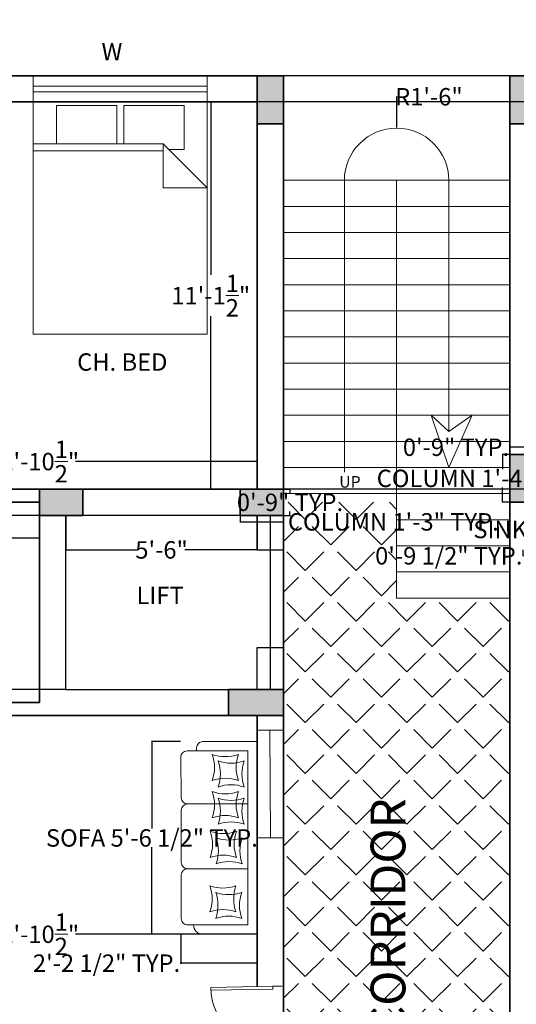
# Model space of a CAD drawing. Units: inches. Extents: x -2181 to 1225, y -80 to 4016.
# Tile 4 of 10: x 497 to 668, y 253 to 592. Entities that reach past the tile are written whole.
import ezdxf

# ---------------------------------------------------------------- set-up
doc = ezdxf.new("R2010")
doc.units = ezdxf.units.IN
doc.header["$MEASUREMENT"] = 0
for name, color, linetype, lineweight in [('A-ANNO-DIMS', 2, 'Continuous', 18), ('A-ANNO-TEXT', 7, 'Continuous', 18), ('A-AREA-IDEN', 7, 'Continuous', 18), ('A-COLS', 7, 'Continuous', 35), ('A-COLS-PATT', 252, 'Continuous', 13), ('A-DOOR', 3, 'Continuous', 18), ('A-FLOR', 7, 'Continuous', 25), ('A-FLOR-EVTR', 7, 'Continuous', 25), ('A-FLOR-PATT', 252, 'Continuous', 13), ('A-FLOR-STRS', 7, 'Continuous', 18), ('A-FURN', 30, 'Continuous', 18), ('A-GLAZ', 4, 'Continuous', 18), ('A-WALL', 7, 'Continuous', 35)]:
    doc.layers.add(name, color=color, linetype=linetype, lineweight=lineweight)
doc.styles.get("Standard").update_dxf_attribs({"font": 'arial.ttf'})
doc.dimstyles.get("Standard").update_dxf_attribs({"dimtxt": 6, "dimasz": 0.18, "dimexe": 0.18, "dimexo": 0.0625, "dimgap": 0.09, "dimtad": 0, "dimtih": 1, "dimtoh": 1, "dimdec": 4, "dimzin": 0, "dimdsep": 46, "dimlunit": 4, "dimtxsty": 'Standard', "dimcen": 0.09, "dimadec": 0, "dimazin": 0, "dimtfac": 1, "dimtdec": 4, "dimtofl": 0, "dimtmove": 0, "dimatfit": 3, "dimfxl": 1, "dimtolj": 1, "dimtzin": 0, "dimarcsym": 0})

# ---------------------------------------------------------------- blocks, each defined once
blk = doc.blocks.new('*U2')
for p, q in [((0, 0), (0, -6)), ((40, 0), (40, -6))]:
    blk.add_line(p, q)
blk.add_lwpolyline([(0, 0), (0, 40), (1.75, 40), (1.75, 0)], close=True)
blk.add_arc((0, 0), 40, 0, 90)
blk = doc.blocks.new('Bed - Queen')
for p, q in [((0, -80.00003), (0, 0)), ((0, 0), (59.99999, 0)), ((59.99999, 0), (59.99999, -80.00003)), ((7.99999, -1.2), (28.79998, -1.2)), ((7.99999, -14.4), (7.99999, -1.2)), ((28.79998, -1.2), (28.79998, -14.4)), ((31.19999, -1.2), (51.99999, -1.2)), ((31.19999, -14.4), (31.19999, -1.2)), ((51.99999, -1.2), (51.99999, -16.4)), ((0, -14.4), (44.8, -14.4)), ((44.8, -16.8), (0, -16.8)), ((59.99999, -29.6), (44.8, -14.4)), ((44.8, -14.4), (44.8, -29.6)), ((51.99999, -16.4), (46.79936, -16.4)), ((44.8, -29.6), (59.99999, -29.6)), ((59.99999, -80.00003), (0, -80.00003))]:
    blk.add_line(p, q)
blk = doc.blocks.new('*D22')
at = {"layer": 'A-ANNO-DIMS', "color": 0, "lineweight": -2, "transparency": 16777216}
for p, q in [((470.02, 664.48), (474.9, 664.48)), ((474.72, 664.3), (474.72, 625.85)), ((474.72, 573.16), (474.72, 611.62)), ((624.01, 572.98), (474.54, 572.98))]:
    blk.add_line(p, q, dxfattribs=at)
at = {"layer": 'A-ANNO-DIMS', "color": 0, "transparency": 16777216}
for points in [[(474.69, 664.3), (474.75, 664.3), (474.72, 664.48)], [(474.69, 573.16), (474.75, 573.16), (474.72, 572.98)]]:
    blk.add_solid(points, dxfattribs=at)
at = {"layer": 'Defpoints', "color": 0, "transparency": 16777216}
for p in [(469.95, 664.48), (474.72, 572.98), (624.08, 572.98)]:
    blk.add_point(p, dxfattribs=at)
at = {"layer": 'A-ANNO-DIMS', "color": 0, "transparency": 16777216, "insert": (474.72, 618.73), "char_height": 6, "attachment_point": 5}
blk.add_mtext('\\A1;7\'-7{\\H1x;\\S1/2;}"', dxfattribs=at)
blk = doc.blocks.new('*D43')
at = {"layer": 'A-ANNO-DIMS', "color": 0, "lineweight": -2, "transparency": 16777216}
for p, q in [((424.01, 281.17), (424.01, 276.89)), ((424.19, 277.07), (486.63, 277.07)), ((578.33, 277.07), (515.9, 277.07)), ((578.51, 277.13), (578.51, 277.25))]:
    blk.add_line(p, q, dxfattribs=at)
at = {"layer": 'A-ANNO-DIMS', "color": 0, "transparency": 16777216}
for points in [[(424.19, 277.1), (424.19, 277.04), (424.01, 277.07)], [(578.33, 277.1), (578.33, 277.04), (578.51, 277.07)]]:
    blk.add_solid(points, dxfattribs=at)
at = {"layer": 'Defpoints', "color": 0, "transparency": 16777216}
for p in [(424.01, 281.23), (578.51, 277.07), (578.51, 277.07)]:
    blk.add_point(p, dxfattribs=at)
at = {"layer": 'A-ANNO-DIMS', "color": 0, "transparency": 16777216, "insert": (501.26, 277.07), "char_height": 6, "attachment_point": 5}
blk.add_mtext('\\A1;12\'-10{\\H1x;\\S1/2;}"', dxfattribs=at)
blk = doc.blocks.new('*D45')
at = {"layer": 'A-ANNO-DIMS', "color": 0, "lineweight": -2, "transparency": 16777216}
for p, q in [((449.01, 425.92), (449.01, 413.4)), ((503.46, 425.92), (503.46, 413.4)), ((449.19, 413.58), (469.45, 413.58)), ((503.28, 413.58), (483.03, 413.58))]:
    blk.add_line(p, q, dxfattribs=at)
at = {"layer": 'A-ANNO-DIMS', "color": 0, "transparency": 16777216}
for points in [[(449.19, 413.61), (449.19, 413.55), (449.01, 413.58)], [(503.28, 413.61), (503.28, 413.55), (503.46, 413.58)]]:
    blk.add_solid(points, dxfattribs=at)
at = {"layer": 'Defpoints', "color": 0, "transparency": 16777216}
for p in [(449.01, 425.98), (503.46, 425.98), (503.46, 413.58)]:
    blk.add_point(p, dxfattribs=at)
at = {"layer": 'A-ANNO-DIMS', "color": 0, "transparency": 16777216, "insert": (476.24, 413.58), "char_height": 6, "width": 24.618, "attachment_point": 5}
blk.add_mtext('\\A1;4\'6"', dxfattribs=at)
blk = doc.blocks.new('*D46')
at = {"layer": 'A-ANNO-DIMS', "color": 0, "lineweight": -2, "transparency": 16777216}
for p, q in [((512.51, 421.42), (512.51, 409.39)), ((578.51, 421.42), (578.51, 409.39)), ((512.69, 409.57), (537.45, 409.57)), ((578.33, 409.57), (553.58, 409.57))]:
    blk.add_line(p, q, dxfattribs=at)
at = {"layer": 'A-ANNO-DIMS', "color": 0, "transparency": 16777216}
for points in [[(512.69, 409.6), (512.69, 409.54), (512.51, 409.57)], [(578.33, 409.6), (578.33, 409.54), (578.51, 409.57)]]:
    blk.add_solid(points, dxfattribs=at)
at = {"layer": 'Defpoints', "color": 0, "transparency": 16777216}
for p in [(512.51, 421.48), (578.51, 421.48), (578.51, 409.57)]:
    blk.add_point(p, dxfattribs=at)
at = {"layer": 'A-ANNO-DIMS', "color": 0, "transparency": 16777216, "insert": (545.51, 409.57), "char_height": 6, "attachment_point": 5}
blk.add_mtext('\\A1;5\'-6"', dxfattribs=at)
blk = doc.blocks.new('*D47')
at = {"layer": 'A-ANNO-DIMS', "color": 0, "lineweight": -2, "transparency": 16777216}
for p, q in [((578.45, 563.98), (562.29, 563.98)), ((562.47, 563.8), (562.47, 504.35)), ((562.47, 430.66), (562.47, 490.12)), ((578.45, 430.48), (562.29, 430.48))]:
    blk.add_line(p, q, dxfattribs=at)
at = {"layer": 'A-ANNO-DIMS', "color": 0, "transparency": 16777216}
for points in [[(562.44, 563.8), (562.5, 563.8), (562.47, 563.98)], [(562.44, 430.66), (562.5, 430.66), (562.47, 430.48)]]:
    blk.add_solid(points, dxfattribs=at)
at = {"layer": 'Defpoints', "color": 0, "transparency": 16777216}
for p in [(578.51, 563.98), (562.47, 430.48), (578.51, 430.48)]:
    blk.add_point(p, dxfattribs=at)
at = {"layer": 'A-ANNO-DIMS', "color": 0, "transparency": 16777216, "insert": (562.47, 497.23), "char_height": 6, "attachment_point": 5}
blk.add_mtext('\\A1;11\'-1{\\H1x;\\S1/2;}"', dxfattribs=at)
blk = doc.blocks.new('*D48')
at = {"layer": 'A-ANNO-DIMS', "color": 0, "lineweight": -2, "transparency": 16777216}
for p, q in [((424.01, 430.55), (424.01, 440.19)), ((424.19, 440.01), (486.63, 440.01)), ((578.33, 440.01), (515.9, 440.01)), ((578.51, 430.55), (578.51, 440.19))]:
    blk.add_line(p, q, dxfattribs=at)
at = {"layer": 'A-ANNO-DIMS', "color": 0, "transparency": 16777216}
for points in [[(424.19, 440.04), (424.19, 439.98), (424.01, 440.01)], [(578.33, 440.04), (578.33, 439.98), (578.51, 440.01)]]:
    blk.add_solid(points, dxfattribs=at)
at = {"layer": 'Defpoints', "color": 0, "transparency": 16777216}
for p in [(578.51, 440.01), (424.01, 430.48), (578.51, 430.48)]:
    blk.add_point(p, dxfattribs=at)
at = {"layer": 'A-ANNO-DIMS', "color": 0, "transparency": 16777216, "insert": (501.26, 440.01), "char_height": 6, "attachment_point": 5}
blk.add_mtext('\\A1;12\'-10{\\H1x;\\S1/2;}"', dxfattribs=at)
blk = doc.blocks.new('*D71')
at = {"layer": 'A-ANNO-DIMS', "color": 0, "lineweight": -2, "transparency": 16777216}
for p, q in [((98.51, 573.05), (98.51, 611.58)), ((98.69, 611.4), (536.64, 611.4)), ((995.33, 611.4), (557.39, 611.4)), ((995.51, 573.05), (995.51, 611.58))]:
    blk.add_line(p, q, dxfattribs=at)
at = {"layer": 'A-ANNO-DIMS', "color": 0, "transparency": 16777216}
for points in [[(98.69, 611.43), (98.69, 611.37), (98.51, 611.4)], [(995.33, 611.43), (995.33, 611.37), (995.51, 611.4)]]:
    blk.add_solid(points, dxfattribs=at)
at = {"layer": 'Defpoints', "color": 0, "transparency": 16777216}
for p in [(995.51, 611.4), (98.51, 572.98), (995.51, 572.98)]:
    blk.add_point(p, dxfattribs=at)
at = {"layer": 'A-ANNO-DIMS', "color": 0, "transparency": 16777216, "insert": (547.01, 611.4), "char_height": 6, "attachment_point": 5}
blk.add_mtext('\\A1;74\'-9"', dxfattribs=at)
blk = doc.blocks.new('SOFA-UPHOLSTERED')
for p, q in [((3.23, 44.91), (24.04, 44.91)), ((3.23, 22.57), (24.04, 22.58)), ((25.11, 22.58), (25.11, 22.58))]:
    blk.add_line(p, q)
for points in [[(0, 0), (0, 66.42), (18.76, 66.42, -0.414214), (20.91, 64.27), (20.91, 63.19)], [(3.23, 3.23), (3.23, 63.19), (24.21, 63.19, -0.417877), (26.36, 61.02), (26.19, 47.04, -0.410559), (24.04, 44.91), (3.23, 44.91)], [(26.19, 42.76), (26.19, 24.73, -0.414214), (24.04, 22.58), (3.23, 22.58)], [(26.19, 20.43), (26.19, 5.38, -0.414214), (24.04, 3.23), (3.23, 3.23)], [(21.99, 3.23), (21.99, 3.23, -0.414214), (18.76, 0), (0, 0)]]:
    blk.add_lwpolyline(points, format="xyb")
for points in [[(18.76, 66.42), (19, 66.42)], [(19, 0), (18.76, 0)]]:
    blk.add_lwpolyline(points)
for centre, radius, start, end in [((11.03, 74.56), 13.33, 250.2663, 289.7337), ((-6.02, 57.51), 13.33, 340.2663, 19.7337), ((28.07, 57.51), 13.33, 160.2663, 199.7337), ((9.03, 72.31), 13.33, 250.2663, 289.7337), ((-8.02, 55.27), 13.33, 340.2663, 19.7337), ((26.07, 55.27), 13.33, 160.2663, 199.7337), ((9.03, 38.22), 13.33, 70.2663, 109.7337), ((11.03, 40.47), 13.33, 70.2663, 109.7337), ((11.03, 61.71), 13.33, 250.2663, 289.7337), ((-6.02, 44.66), 13.33, 340.2663, 19.7337), ((28.07, 44.66), 13.33, 160.2663, 199.7337), ((9.03, 59.47), 13.33, 250.2663, 289.7337), ((-8.02, 42.42), 13.33, 340.2663, 19.7337), ((26.07, 42.42), 13.33, 160.2663, 199.7337), ((24.04, 42.76), 2.15, 360, 90), ((11.03, 27.62), 13.33, 70.2663, 109.7337), ((9.03, 25.38), 13.33, 70.2663, 109.7337), ((11.72, 48.03), 13.33, 250.2663, 289.7337), ((-5.33, 30.99), 13.33, 340.2663, 19.7337), ((28.76, 30.99), 13.33, 160.2663, 199.7337), ((9.72, 45.79), 13.33, 250.2663, 289.7337), ((-7.33, 28.74), 13.33, 340.2663, 19.7337), ((26.76, 28.74), 13.33, 160.2663, 199.7337), ((11.72, 13.94), 13.33, 70.2663, 109.7337), ((9.72, 11.7), 13.33, 70.2663, 109.7337), ((24.04, 20.43), 2.15, 0, 90.0249), ((9.86, 27), 13.33, 250.2663, 289.7337), ((-7.19, 9.96), 13.33, 340.2663, 19.7337), ((11.86, 29.25), 13.33, 250.2663, 289.7337), ((-5.19, 12.2), 13.33, 340.2663, 19.7337), ((26.9, 9.96), 13.33, 160.2663, 199.7337), ((28.9, 12.2), 13.33, 160.2663, 199.7337), ((11.86, -4.84), 13.33, 70.2663, 109.7337), ((9.86, -7.09), 13.33, 70.2663, 109.7337)]:
    blk.add_arc(centre, radius, start, end)
blk = doc.blocks.new('COL-16.5X9')
blk.add_lwpolyline([(0, 16.5), (9, 16.5), (9, 0), (0, 0)], close=True)
blk = doc.blocks.new('COL-18.89X9')
blk.add_lwpolyline([(18.9, 9), (0, 9), (0, 0), (18.9, 0)], close=True)
blk = doc.blocks.new('COL-14.94X9')
blk.add_lwpolyline([(0, 9), (14.94, 9), (14.94, 0), (0, 0)], close=True)
blk = doc.blocks.new('WIN-60')
for p, q in [((0, 0), (0, 9)), ((60, 0), (60, 9)), ((0, 5.5), (60, 5.5)), ((0, 3.5), (60, 3.5))]:
    blk.add_line(p, q)
blk = doc.blocks.new('*D92')
at = {"layer": 'A-ANNO-DIMS', "color": 0, "lineweight": -2, "transparency": 16777216}
for p, q in [((679.38, 423.59), (681.59, 423.59)), ((681.41, 423.41), (681.41, 419.8)), ((681.41, 409.82), (681.41, 413.42)), ((679.38, 409.64), (681.59, 409.64))]:
    blk.add_line(p, q, dxfattribs=at)
at = {"layer": 'A-ANNO-DIMS', "color": 0, "transparency": 16777216}
for points in [[(681.38, 423.41), (681.44, 423.41), (681.41, 423.59)], [(681.38, 409.82), (681.44, 409.82), (681.41, 409.64)]]:
    blk.add_solid(points, dxfattribs=at)
at = {"layer": 'Defpoints', "color": 0, "transparency": 16777216}
for p in [(679.31, 423.59), (679.31, 409.64), (681.41, 409.64)]:
    blk.add_point(p, dxfattribs=at)
at = {"layer": 'A-ANNO-DIMS', "color": 0, "transparency": 16777216, "insert": (681.41, 416.61), "char_height": 6, "attachment_point": 5}
blk.add_mtext('\\A1;SINK 1\'-2" TYP.', dxfattribs=at)
blk = doc.blocks.new('*D93')
at = {"layer": 'A-ANNO-DIMS', "color": 0, "lineweight": -2, "transparency": 16777216}
for p, q in [((670.01, 407.54), (669.83, 407.54)), ((670.01, 409.57), (670.01, 407.36)), ((679.13, 407.54), (670.19, 407.54)), ((679.31, 409.57), (679.31, 407.36))]:
    blk.add_line(p, q, dxfattribs=at)
at = {"layer": 'A-ANNO-DIMS', "color": 0, "transparency": 16777216}
for points in [[(670.19, 407.57), (670.19, 407.51), (670.01, 407.54)], [(679.13, 407.57), (679.13, 407.51), (679.31, 407.54)]]:
    blk.add_solid(points, dxfattribs=at)
at = {"layer": 'Defpoints', "color": 0, "transparency": 16777216}
for p in [(670.01, 409.64), (670.01, 407.54), (679.31, 409.64)]:
    blk.add_point(p, dxfattribs=at)
at = {"layer": 'A-ANNO-DIMS', "color": 0, "transparency": 16777216, "insert": (644.47, 407.54), "char_height": 6, "attachment_point": 5}
blk.add_mtext('\\A1;0\'-9 1/2" TYP.', dxfattribs=at)
blk = doc.blocks.new('*D104')
at = {"layer": 'A-ANNO-DIMS', "color": 0, "lineweight": -2, "transparency": 16777216}
for p, q in [((665.45, 442.48), (662.86, 442.48)), ((663.04, 442.3), (663.04, 437.43)), ((663.04, 426.16), (663.04, 431.04)), ((665.45, 425.98), (662.86, 425.98))]:
    blk.add_line(p, q, dxfattribs=at)
at = {"layer": 'A-ANNO-DIMS', "color": 0, "transparency": 16777216}
for points in [[(663.01, 442.3), (663.07, 442.3), (663.04, 442.48)], [(663.01, 426.16), (663.07, 426.16), (663.04, 425.98)]]:
    blk.add_solid(points, dxfattribs=at)
at = {"layer": 'Defpoints', "color": 0, "transparency": 16777216}
for p in [(665.51, 442.48), (663.04, 425.98), (665.51, 425.98)]:
    blk.add_point(p, dxfattribs=at)
at = {"layer": 'A-ANNO-DIMS', "color": 0, "transparency": 16777216, "insert": (663.04, 434.23), "char_height": 6, "attachment_point": 5}
blk.add_mtext('\\A1;COLUMN 1\'-4 1/2" TYP.', dxfattribs=at)
blk = doc.blocks.new('*D105')
at = {"layer": 'A-ANNO-DIMS', "color": 0, "lineweight": -2, "transparency": 16777216}
for p, q in [((665.51, 444.96), (665.33, 444.96)), ((665.51, 442.55), (665.51, 445.14)), ((674.33, 444.96), (665.69, 444.96)), ((674.51, 442.55), (674.51, 445.14))]:
    blk.add_line(p, q, dxfattribs=at)
at = {"layer": 'A-ANNO-DIMS', "color": 0, "transparency": 16777216}
for points in [[(665.69, 444.99), (665.69, 444.93), (665.51, 444.96)], [(674.33, 444.99), (674.33, 444.93), (674.51, 444.96)]]:
    blk.add_solid(points, dxfattribs=at)
at = {"layer": 'Defpoints', "color": 0, "transparency": 16777216}
for p in [(665.51, 444.96), (665.51, 442.48), (674.51, 442.48)]:
    blk.add_point(p, dxfattribs=at)
at = {"layer": 'A-ANNO-DIMS', "color": 0, "transparency": 16777216, "insert": (646.96, 444.96), "char_height": 6, "attachment_point": 5}
blk.add_mtext('\\A1;0\'-9" TYP.', dxfattribs=at)
blk = doc.blocks.new('*D106')
at = {"layer": 'A-ANNO-DIMS', "color": 0, "lineweight": -2, "transparency": 16777216}
for p, q in [((552.08, 343.49), (542, 343.49)), ((542.18, 343.31), (542.18, 313.48)), ((542.18, 277.25), (542.18, 307.09)), ((552.08, 277.07), (542, 277.07))]:
    blk.add_line(p, q, dxfattribs=at)
at = {"layer": 'A-ANNO-DIMS', "color": 0, "transparency": 16777216}
for points in [[(542.15, 343.31), (542.21, 343.31), (542.18, 343.49)], [(542.15, 277.25), (542.21, 277.25), (542.18, 277.07)]]:
    blk.add_solid(points, dxfattribs=at)
at = {"layer": 'Defpoints', "color": 0, "transparency": 16777216}
for p in [(542.18, 343.49), (552.14, 343.49), (552.14, 277.07)]:
    blk.add_point(p, dxfattribs=at)
at = {"layer": 'A-ANNO-DIMS', "color": 0, "transparency": 16777216, "insert": (542.18, 310.28), "char_height": 6, "attachment_point": 5}
blk.add_mtext('\\A1;SOFA 5\'-6 1/2" TYP.', dxfattribs=at)
blk = doc.blocks.new('*D107')
at = {"layer": 'A-ANNO-DIMS', "color": 0, "lineweight": -2, "transparency": 16777216}
for p, q in [((552.14, 277.01), (552.14, 266.93)), ((578.51, 277.01), (578.51, 266.93)), ((552.14, 267.11), (551.96, 267.11)), ((578.33, 267.11), (552.32, 267.11))]:
    blk.add_line(p, q, dxfattribs=at)
at = {"layer": 'A-ANNO-DIMS', "color": 0, "transparency": 16777216}
for points in [[(552.32, 267.14), (552.32, 267.08), (552.14, 267.11)], [(578.33, 267.14), (578.33, 267.08), (578.51, 267.11)]]:
    blk.add_solid(points, dxfattribs=at)
at = {"layer": 'Defpoints', "color": 0, "transparency": 16777216}
for p in [(552.14, 277.07), (578.51, 277.07), (552.14, 267.11)]:
    blk.add_point(p, dxfattribs=at)
at = {"layer": 'A-ANNO-DIMS', "color": 0, "transparency": 16777216, "insert": (526.55, 267.11), "char_height": 6, "attachment_point": 5}
blk.add_mtext('\\A1;2\'-2 1/2" TYP.', dxfattribs=at)
blk = doc.blocks.new('*D118')
at = {"layer": 'A-ANNO-DIMS', "color": 0, "lineweight": -2, "transparency": 16777216}
for p, q in [((572.57, 421.42), (572.57, 419.06)), ((587.51, 421.42), (587.51, 419.06)), ((572.75, 419.24), (587.33, 419.24)), ((587.51, 419.24), (587.69, 419.24))]:
    blk.add_line(p, q, dxfattribs=at)
at = {"layer": 'A-ANNO-DIMS', "color": 0, "transparency": 16777216}
for points in [[(572.75, 419.27), (572.75, 419.21), (572.57, 419.24)], [(587.33, 419.27), (587.33, 419.21), (587.51, 419.24)]]:
    blk.add_solid(points, dxfattribs=at)
at = {"layer": 'Defpoints', "color": 0, "transparency": 16777216}
for p in [(572.57, 421.48), (587.51, 421.48), (587.51, 419.24)]:
    blk.add_point(p, dxfattribs=at)
at = {"layer": 'A-ANNO-DIMS', "color": 0, "transparency": 16777216, "insert": (625.36, 419.24), "char_height": 6, "attachment_point": 5}
blk.add_mtext('\\A1;COLUMN 1\'-3" TYP.', dxfattribs=at)
blk = doc.blocks.new('*D119')
at = {"layer": 'A-ANNO-DIMS', "color": 0, "lineweight": -2, "transparency": 16777216}
for p, q in [((587.58, 430.48), (589.94, 430.48)), ((589.76, 430.3), (589.76, 429.14)), ((587.58, 421.48), (589.94, 421.48)), ((589.76, 421.66), (589.76, 422.83))]:
    blk.add_line(p, q, dxfattribs=at)
at = {"layer": 'A-ANNO-DIMS', "color": 0, "transparency": 16777216}
for points in [[(589.73, 430.3), (589.79, 430.3), (589.76, 430.48)], [(589.73, 421.66), (589.79, 421.66), (589.76, 421.48)]]:
    blk.add_solid(points, dxfattribs=at)
at = {"layer": 'Defpoints', "color": 0, "transparency": 16777216}
for p in [(587.51, 430.48), (589.76, 430.48), (587.51, 421.48)]:
    blk.add_point(p, dxfattribs=at)
at = {"layer": 'A-ANNO-DIMS', "color": 0, "transparency": 16777216, "insert": (589.76, 425.98), "char_height": 6, "attachment_point": 5}
blk.add_mtext('\\A1;0\'-9" TYP.', dxfattribs=at)
blk = doc.blocks.new('*D130')
at = {"layer": 'A-ANNO-DIMS', "color": 0, "lineweight": -2, "transparency": 16777216}
for p, q in [((512.45, 421.48), (-59.44, 421.48)), ((-59.26, 421.3), (-59.26, 394.64)), ((-59.26, 361.66), (-59.26, 388.33)), ((512.45, 361.48), (-59.44, 361.48))]:
    blk.add_line(p, q, dxfattribs=at)
at = {"layer": 'A-ANNO-DIMS', "color": 0, "transparency": 16777216}
for points in [[(-59.29, 421.3), (-59.23, 421.3), (-59.26, 421.48)], [(-59.29, 361.66), (-59.23, 361.66), (-59.26, 361.48)]]:
    blk.add_solid(points, dxfattribs=at)
at = {"layer": 'Defpoints', "color": 0, "transparency": 16777216}
for p in [(512.51, 421.48), (-59.26, 361.48), (512.51, 361.48)]:
    blk.add_point(p, dxfattribs=at)
at = {"layer": 'A-ANNO-DIMS', "color": 0, "transparency": 16777216, "insert": (-59.26, 391.48), "char_height": 6, "attachment_point": 5}
blk.add_mtext('\\A1;5\'-0"', dxfattribs=at)
blk = doc.blocks.new('*D131')
at = {"layer": 'A-ANNO-DIMS', "color": 0, "lineweight": -2, "transparency": 16777216}
for p, q in [((976.64, 563.98), (-59.44, 563.98)), ((-59.26, 563.8), (-59.26, 500.43)), ((-59.26, 430.66), (-59.26, 494.04)), ((977.45, 430.48), (-59.44, 430.48))]:
    blk.add_line(p, q, dxfattribs=at)
at = {"layer": 'A-ANNO-DIMS', "color": 0, "transparency": 16777216}
for points in [[(-59.29, 563.8), (-59.23, 563.8), (-59.26, 563.98)], [(-59.29, 430.66), (-59.23, 430.66), (-59.26, 430.48)]]:
    blk.add_solid(points, dxfattribs=at)
at = {"layer": 'Defpoints', "color": 0, "transparency": 16777216}
for p in [(976.7, 563.98), (-59.26, 430.48), (977.51, 430.48)]:
    blk.add_point(p, dxfattribs=at)
at = {"layer": 'A-ANNO-DIMS', "color": 0, "transparency": 16777216, "insert": (-59.26, 497.23), "char_height": 6, "attachment_point": 5}
blk.add_mtext('\\A1;11\'-1 1/2"', dxfattribs=at)
blk = doc.blocks.new('*D135')
at = {"layer": 'A-ANNO-DIMS', "color": 0, "lineweight": -2, "transparency": 16777216}
for p, q in [((626.7, 565.78), (626.52, 565.78)), ((626.52, 565.78), (626.51, 555.16)), ((626.42, 536.98), (626.6, 536.98)), ((626.51, 536.89), (626.51, 537.07))]:
    blk.add_line(p, q, dxfattribs=at)
at = {"layer": 'A-ANNO-DIMS', "color": 0, "transparency": 16777216}
blk.add_solid([(626.49, 555.16), (626.55, 555.16), (626.51, 554.98)], dxfattribs=at)
at = {"layer": 'Defpoints', "color": 0, "transparency": 16777216}
for p in [(626.51, 554.98), (626.51, 536.98)]:
    blk.add_point(p, dxfattribs=at)
at = {"layer": 'A-ANNO-DIMS', "color": 0, "transparency": 16777216, "insert": (637.63, 565.78), "char_height": 6, "attachment_point": 5}
blk.add_mtext('\\A1;R1\'-6"', dxfattribs=at)

msp = doc.modelspace()

# ---------------------------------------------------------------- hatches: boundary and pattern name
at = {"layer": 'A-COLS-PATT'}
h = msp.add_hatch(color=256, dxfattribs=at)
h.dxf.hatch_style = 1
h.paths.add_polyline_path([(587.51461, 572.98479), (578.51461, 572.98479), (578.51461, 556.48479), (587.51461, 556.48479)])
h = msp.add_hatch(color=256, dxfattribs=at)
h.dxf.hatch_style = 1
h.paths.add_polyline_path([(995.51461, 209.98479), (986.51461, 209.98479), (986.51461, 191.48479), (995.51461, 191.48479)])
h.paths.add_polyline_path([(862.50488, 191.48479), (862.50488, 200.48479), (841.01461, 200.48479), (841.01461, 191.48479)])
h.paths.add_polyline_path([(995.51461, 425.98479), (995.51461, 434.98479), (977.51461, 434.98479), (977.51461, 425.98479)])
h.paths.add_polyline_path([(880.01461, 425.98479), (880.01461, 432.54138), (862.01461, 432.54138), (862.01461, 425.98479)])
h.paths.add_polyline_path([(880.82546, 563.98479), (880.82546, 572.98479), (862.01461, 572.98479), (862.01461, 563.98479)])
h.paths.add_polyline_path([(995.51461, 563.98479), (995.51461, 572.98479), (976.70377, 572.98479), (976.70377, 563.98479)])
h.paths.add_polyline_path([(674.51461, 572.98479), (665.51461, 572.98479), (665.51461, 556.48479), (674.51461, 556.48479)])
h.paths.add_polyline_path([(674.51461, 442.48479), (665.51461, 442.48479), (665.51461, 425.98479), (674.51461, 425.98479)])
h = msp.add_hatch(color=256, dxfattribs=at)
h.dxf.hatch_style = 1
h.paths.add_polyline_path([(269.21166, 145.48479), (269.21166, 136.48479), (297.04101, 136.48479), (297.04101, 145.48479)])
h.paths.add_polyline_path([(445.01461, 352.48479), (445.01461, 361.48479), (426.1199, 361.48479), (426.1199, 352.48479)])
h.paths.add_polyline_path([(587.51461, 352.48479), (587.51461, 361.48479), (568.6199, 361.48479), (568.6199, 352.48479)])
h.paths.add_polyline_path([(518.40498, 421.48479), (518.40498, 430.48479), (503.51461, 430.48479), (503.51461, 421.48479)])
h.paths.add_polyline_path([(587.51461, 421.48479), (587.51461, 430.48479), (572.5711, 430.48479), (572.5711, 421.48479)])
at = {"layer": 'A-FLOR-PATT'}
h = msp.add_hatch(dxfattribs=at)
h.set_pattern_fill('ANGLE', color=256, scale=45, angle=45)
h.set_pattern_definition([(45, (0, 0), (-8.75045, 8.75045), [9, -3.375]), (135, (0, 0), (-8.75045, -8.75045), [9, -3.375])])
h.paths.add_polyline_path([(626.51461, 392.98479), (626.51461, 425.98479), (587.51461, 425.98479), (587.51461, 137.48479), (665.51461, 137.48479), (665.51461, 392.98479)])

# ---------------------------------------------------------------- linework, layer by layer
at = {"layer": 'A-FLOR'}
msp.add_lwpolyline([(665.51461, 572.98479), (587.51461, 572.98479)], dxfattribs=at)
at = {"layer": 'A-FLOR-EVTR'}
for p, q in [((578.51461, 409.57464), (587.51461, 409.57464)), ((578.51461, 375.94958), (587.51461, 375.94958))]:
    msp.add_line(p, q, dxfattribs=at)
for points in [[(512.51461, 361.48479), (512.51461, 421.48479)], [(587.51461, 421.48479), (512.51461, 421.48479)], [(578.51461, 409.57464), (578.51461, 421.48479)], [(583.01461, 361.48479), (583.01461, 421.48479)], [(578.51461, 361.48479), (578.51461, 375.94958)], [(512.51461, 361.48479), (578.51461, 361.48479)]]:
    msp.add_lwpolyline(points, dxfattribs=at)
at = {"layer": 'A-FLOR-STRS'}
for p, q in [((608.51461, 436.35434), (608.51461, 536.98479)), ((626.51461, 437.98479), (626.51461, 536.98479)), ((644.51461, 450.36751), (644.51461, 536.98479)), ((644.51461, 437.98479), (638.37985, 455.98479)), ((638.37985, 455.98479), (644.51461, 437.98479)), ((638.37985, 455.98479), (644.51461, 450.36751)), ((644.51461, 437.98479), (652.55128, 455.98479)), ((644.51461, 450.36751), (652.55128, 455.98479)), ((626.51461, 392.98479), (626.51461, 437.98479))]:
    msp.add_line(p, q, dxfattribs=at)
for points in [[(665.51461, 536.98479), (587.51461, 536.98479)], [(665.51461, 527.98479), (587.51461, 527.98479)], [(665.51461, 518.98479), (587.51461, 518.98479)], [(665.51461, 509.98479), (587.51461, 509.98479)], [(665.51461, 500.98479), (587.51461, 500.98479)], [(665.51461, 491.98479), (587.51461, 491.98479)], [(665.51461, 482.98479), (587.51461, 482.98479)], [(665.51461, 473.98479), (587.51461, 473.98479)], [(665.51461, 464.98479), (587.51461, 464.98479)], [(665.51461, 455.98479), (587.51461, 455.98479)], [(665.51461, 446.98479), (587.51461, 446.98479)], [(665.51461, 437.98479), (587.51461, 437.98479)], [(665.51461, 428.98479), (587.51461, 428.98479)], [(665.51461, 419.98479), (626.51461, 419.98479)], [(665.51461, 410.98479), (626.51461, 410.98479)], [(665.51461, 401.98479), (626.51461, 401.98479)], [(665.51461, 392.98479), (626.51461, 392.98479)]]:
    msp.add_lwpolyline(points, dxfattribs=at)
msp.add_arc((626.51461, 536.98479), 18, 0, 180, dxfattribs=at)
at = {"layer": 'A-GLAZ'}
for p, q in [((578.51461, 347.38534), (587.51461, 347.38534)), ((583.01461, 310.28152), (582.80601, 347.38534)), ((578.51461, 310.28152), (587.51461, 310.28152))]:
    msp.add_line(p, q, dxfattribs=at)
at = {"layer": 'A-WALL'}
for points in [[(587.51461, 572.98479), (98.51461, 572.98479), (98.51461, 136.48479)], [(587.51461, 136.48479), (587.51461, 572.98479)], [(995.51461, 136.48479), (995.51461, 572.98479), (665.51461, 572.98479)], [(665.51461, 136.48479), (665.51461, 572.98479)], [(578.51461, 563.98479), (419.51461, 563.98479)], [(578.51461, 563.98479), (424.01461, 563.98479)], [(578.51461, 430.48479), (578.51461, 563.98479)], [(587.51461, 430.48479), (424.01461, 430.48479)], [(503.51461, 356.98479), (503.51461, 430.48479)], [(503.51461, 425.98479), (449.51461, 425.98479)], [(693.94574, 425.98479), (665.51461, 425.98479)], [(503.51461, 356.98479), (449.01461, 356.98479)], [(445.01461, 352.48479), (578.51461, 352.48479)], [(578.51461, 259.02696), (578.51461, 352.48479)]]:
    msp.add_lwpolyline(points, dxfattribs=at)

# ---------------------------------------------------------------- block references
at = {"layer": 'A-COLS'}
for name, p in [('COL-16.5X9', (578.515, 556.485)), ('COL-16.5X9', (665.515, 556.485)), ('COL-14.94X9', (572.571, 421.485))]:
    msp.add_blockref(name, p, dxfattribs=at)
at = {"layer": 'A-COLS', "rotation": 180}
for name, p in [('COL-16.5X9', (674.51423, 442.48457)), ('COL-18.89X9', (587.51502, 361.48457))]:
    msp.add_blockref(name, p, dxfattribs=at)
at = {"layer": 'A-COLS', "extrusion": (0, 0, -1), "zscale": -1}
msp.add_blockref('COL-14.94X9', (-518.40508, 421.485), dxfattribs=at)
at = {"layer": 'A-DOOR', "extrusion": (0, 0, -1), "xscale": 0.5349745226309166, "yscale": 0.5349745226309166, "zscale": -0.5349745226309166, "rotation": 268.8437329844228}
msp.add_blockref('*U2', (-583.8736, 259.13512), dxfattribs=at)
at = {"layer": 'A-FURN'}
msp.add_blockref('Bed - Queen', (501.26461, 563.98479), dxfattribs=at)
at = {"layer": 'A-FURN', "extrusion": (0, 0, -1), "zscale": -1}
msp.add_blockref('SOFA-UPHOLSTERED', (-578.51476, 277.07219), dxfattribs=at)
at = {"layer": 'A-GLAZ'}
msp.add_blockref('WIN-60', (501.26501, 563.985), dxfattribs=at)

# ---------------------------------------------------------------- texts
at = {"layer": 'A-ANNO-TEXT', "attachment_point": 1}
for s, width, insert, char_height in [('W', 291.4178321, (524.82496, 584.31487), 6), ('UP', 9.9941289, (606.72232, 435.02101), 4)]:
    msp.add_mtext_dynamic_manual_height_columns(s, width=width, gutter_width=1, heights=[0], dxfattribs=dict(at, insert=insert, char_height=char_height))
at = {"layer": 'A-AREA-IDEN', "char_height": 6, "attachment_point": 1}
for s, insert in [('CH. BED', (516.42047, 477.33199)), ('LIFT', (536.88884, 396.88448))]:
    msp.add_mtext_dynamic_manual_height_columns(s, width=291.4178321, gutter_width=1, heights=[0], dxfattribs=dict(at, insert=insert))
at = {"layer": 'A-AREA-IDEN', "insert": (617.54393, 189.77481), "char_height": 12, "attachment_point": 1, "rotation": 90}
msp.add_mtext_dynamic_manual_height_columns('6\'6" W CORRIDOR', width=291.4178321, gutter_width=1, heights=[0], dxfattribs=at)

# ---------------------------------------------------------------- dimensions: what is measured, and where the dimension line sits
at = {"layer": 'A-ANNO-DIMS'}
for base, p1, p2, override, picture, middle in [((474.72038, 572.98479), (469.95283, 664.48479), (624.07639, 572.98479), {"dimclrd": 0, "dimclre": 0, "dimclrt": 0}, '*D22', (474.72038, 618.73479)), ((-59.2566, 430.48478), (976.70377, 563.98478), (977.51461, 430.48478), {"dimdec": 1, "dimlfac": 1, "dimrnd": 0, "dimzin": 1, "dimdsep": 46, "dimlunit": 4, "dimfrac": 2}, '*D131', (-59.2566, 497.23478)), ((562.46823, 430.48479), (578.51461, 563.98479), (578.51461, 430.48479), {"dimclrd": 0, "dimclre": 0, "dimclrt": 0}, '*D47', (562.46823, 497.23479)), ((-59.2566, 361.48478), (512.51461, 421.48478), (512.51461, 361.48478), {"dimdec": 1, "dimlfac": 1, "dimrnd": 0, "dimzin": 1, "dimdsep": 46, "dimlunit": 4, "dimfrac": 2}, '*D130', (-59.2566, 391.48478))]:
    dim = msp.add_linear_dim(base=base, p1=p1, p2=p2, angle=90, dimstyle='Standard', override=override, dxfattribs=at)
    dim.commit()
    dim.dimension.update_dxf_attribs({"geometry": picture, "text_midpoint": middle})
for base, p1, p2, picture, middle in [((995.51461, 611.40365), (98.51461, 572.98479), (995.51461, 572.98479), '*D71', (547.01461, 611.40365)), ((578.51461, 440.00848), (424.01461, 430.48479), (578.51461, 430.48479), '*D48', (501.26461, 440.00848)), ((578.51461, 409.57464), (512.51461, 421.48479), (578.51461, 421.48479), '*D46', (545.51461, 409.57464)), ((578.51461, 277.07243), (424.01461, 281.23479), (578.51461, 277.07243), '*D43', (501.26461, 277.07243))]:
    dim = msp.add_linear_dim(base=base, p1=p1, p2=p2, dimstyle='Standard', override={"dimclrd": 0, "dimclre": 0, "dimclrt": 0}, dxfattribs=at)
    dim.commit()
    dim.dimension.update_dxf_attribs({"geometry": picture, "text_midpoint": middle})
dim = msp.add_radius_dim(center=(626.51461, 536.98478), mpoint=(626.515, 554.98478), dimstyle='Standard', override={"dimdec": 1, "dimlfac": 1, "dimrnd": 0, "dimzin": 1, "dimdsep": 46, "dimlunit": 4, "dimfrac": 2}, dxfattribs=at)
dim.commit()
dim.dimension.update_dxf_attribs({"geometry": '*D135', "text_midpoint": (637.63107, 565.78478), "dimtype": 164})
for base, p1, p2, angle, text, picture, middle in [((663.03961, 425.98479), (665.51461, 442.48479), (665.51461, 425.98479), 270, 'COLUMN <> TYP.', '*D104', (663.03961, 434.23479)), ((665.51461, 444.95979), (674.51461, 442.48479), (665.51461, 442.48479), 180, '<> TYP.', '*D105', (646.95812, 444.95979)), ((589.75614, 430.48479), (587.51461, 421.48479), (587.51461, 430.48479), 90, '<> TYP.', '*D119', (589.75614, 425.98479)), ((681.40622, 409.6364), (679.31389, 423.58532), (679.31389, 409.6364), 270, 'SINK <> TYP.', '*D92', (681.40622, 416.61086)), ((670.01461, 407.54407), (679.31389, 409.6364), (670.01461, 409.6364), 180, '<> TYP.', '*D93', (644.46767, 407.54407)), ((542.18139, 343.49061), (552.14412, 277.07243), (552.14412, 343.49061), 90, 'SOFA <> TYP.', '*D106', (542.18139, 310.28152)), ((552.14412, 267.1097), (578.51461, 277.07243), (552.14412, 277.07243), 180, '<> TYP.', '*D107', (526.54601, 267.1097))]:
    dim = msp.add_linear_dim(base=base, p1=p1, p2=p2, angle=angle, text=text, dimstyle='Standard', override={"dimdec": 1, "dimlfac": 1, "dimrnd": 0, "dimzin": 1, "dimdsep": 46, "dimlunit": 4, "dimfrac": 2}, dxfattribs=at)
    dim.commit()
    dim.dimension.update_dxf_attribs({"geometry": picture, "text_midpoint": middle})
for base, p1, p2, text, override, picture, middle in [((587.51461, 419.24326), (572.5711, 421.48479), (587.51461, 421.48479), 'COLUMN <> TYP.', {"dimdec": 1, "dimlfac": 1, "dimrnd": 0, "dimzin": 1, "dimdsep": 46, "dimlunit": 4, "dimfrac": 2}, '*D118', (625.36238, 419.24326)), ((503.46147, 413.57545), (449.01461, 425.98479), (503.46147, 425.98479), '4\'6"', {"dimclrd": 0, "dimclre": 0, "dimclrt": 0}, '*D45', (476.23804, 413.57545))]:
    dim = msp.add_linear_dim(base=base, p1=p1, p2=p2, text=text, dimstyle='Standard', override=override, dxfattribs=at)
    dim.commit()
    dim.dimension.update_dxf_attribs({"geometry": picture, "text_midpoint": middle})

doc.saveas('drawing.dxf')
